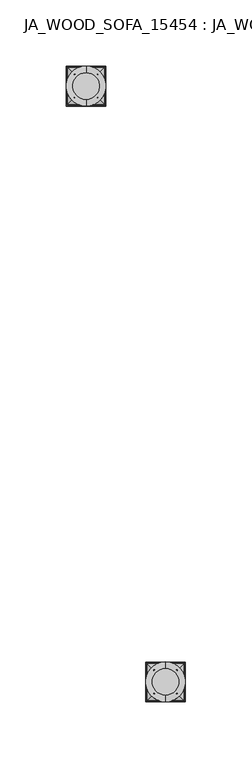
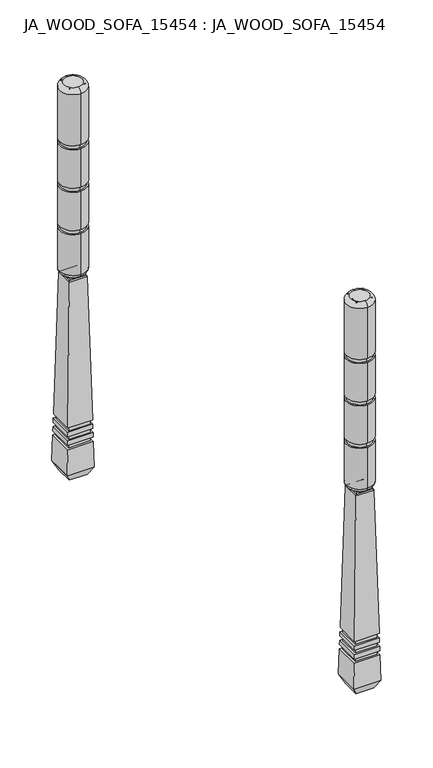
"""IFC4 building model written with IfcOpenShell, lengths in millimetres: furniture geometry, JA_WOOD_SOFA_15454 : JA_WOOD_SOFA_15454."""

from ifc_helpers import new_model, si_unit, point, frame, origin, origin_with_axes, place, context, project, spatial, polyline, circle_curve, ellipse_curve, trimmed, outline, extrude, faceted_brep, source, transform, mapped, element, save
from ifc_brep_helpers import plane_surface, cylinder_surface, revolved_surface, advanced_brep


def ja_wood_sofa_15454_ja_wood_sofa_15454_5725a5a5(model_context):
    return source(origin(), model_context, "Body", "SolidModel", [
        advanced_brep(
        [(237.5, 460.0, 460.0), (237.5, 440.0, 460.0), (237.5, 442.0710678, 235.0), (237.5, 457.9289322, 235.0), (237.5, 465.0, 245.0), (237.5, 465.0, 242.0710678), (237.5, 435.0, 242.0710678), (237.5, 435.0, 245.0), (237.5, 435.0, 290.0), (237.5, 465.0, 290.0), (237.5, 465.0, 455.0000045), (237.5, 465.0, 450.0), (237.5, 465.0, 395.0), (237.5, 435.0, 395.0), (237.5, 435.0, 450.0), (237.5, 435.0, 455.0000074), (237.5, 465.0, 390.0), (237.5, 465.0, 345.0), (237.5, 435.0, 345.0), (237.5, 435.0, 390.0), (237.5, 465.0, 340.0), (237.5, 465.0, 295.0), (237.5, 435.0, 295.0), (237.5, 435.0, 340.0), (237.5, 436.4644661, 238.5355339), (237.5, 463.5355339, 238.5355339), (237.5, 461.4644661, 236.4644661), (237.5, 438.5355339, 236.4644661), (237.5, 437.0, 340.0), (237.5, 437.0, 345.0), (237.5, 463.0, 345.0), (237.5, 463.0, 340.0), (237.5, 437.0, 390.0), (237.5, 437.0, 395.0), (237.5, 463.0, 395.0), (237.5, 463.0, 390.0), (237.5, 437.0, 290.0), (237.5, 437.0, 295.0), (237.5, 463.0, 295.0), (237.5, 463.0, 290.0)],
        [
            (0, 1, circle_curve(frame((237.5, 450.0, 460.0), z_axis=(0.0, 0.0, 1.0), x_axis=(0.0, 1.0, 0.0)), 10.0)),
            (1, 0, circle_curve(frame((237.5, 450.0, 460.0), z_axis=(0.0, 0.0, 1.0), x_axis=(0.0, -1.0, 0.0)), 10.0)),
            (2, 3, circle_curve(frame((237.5, 450.0, 235.0), z_axis=(0.0, 0.0, -1.0), x_axis=(0.0, 1.0, 0.0)), 7.9289322)),
            (3, 2, circle_curve(frame((237.5, 450.0, 235.0), z_axis=(0.0, 0.0, -1.0), x_axis=(0.0, -1.0, 0.0)), 7.9289322)),
            (4, 5),
            (5, 6, circle_curve(frame((237.5, 450.0, 242.0710678), z_axis=(0.0, 0.0, 1.0), x_axis=(0.0, -1.0, 0.0)), 15.0)),
            (6, 7),
            (7, 8),
            (8, 9, circle_curve(frame((237.5, 450.0, 290.0), z_axis=(0.0, 0.0, -1.0), x_axis=(0.0, -1.0, 0.0)), 15.0)),
            (9, 4),
            (10, 11),
            (11, 12),
            (12, 13, circle_curve(frame((237.5, 450.0, 395.0), z_axis=(0.0, 0.0, 1.0), x_axis=(0.0, -1.0, 0.0)), 15.0)),
            (13, 14),
            (14, 15),
            (15, 10, circle_curve(frame((237.5, 450.0, 455.0), z_axis=(0.0, 0.0, -1.0), x_axis=(0.0, -1.0, 0.0)), 15.0)),
            (16, 17),
            (17, 18, circle_curve(frame((237.5, 450.0, 345.0), z_axis=(0.0, 0.0, 1.0), x_axis=(0.0, -1.0, 0.0)), 15.0)),
            (18, 19),
            (19, 16, circle_curve(frame((237.5, 450.0, 390.0), z_axis=(0.0, 0.0, -1.0), x_axis=(0.0, -1.0, 0.0)), 15.0)),
            (20, 21),
            (21, 22, circle_curve(frame((237.5, 450.0, 295.0), z_axis=(0.0, 0.0, 1.0), x_axis=(0.0, -1.0, 0.0)), 15.0)),
            (22, 23),
            (23, 20, circle_curve(frame((237.5, 450.0, 340.0), z_axis=(0.0, 0.0, -1.0), x_axis=(0.0, -1.0, 0.0)), 15.0)),
            (9, 8, circle_curve(frame((237.5, 450.0, 290.0), z_axis=(0.0, 0.0, -1.0), x_axis=(0.0, -1.0, 0.0)), 15.0)),
            (6, 5, circle_curve(frame((237.5, 450.0, 242.0710678), z_axis=(0.0, 0.0, 1.0), x_axis=(0.0, -1.0, 0.0)), 15.0)),
            (10, 15, circle_curve(frame((237.5, 450.0, 455.0), z_axis=(0.0, 0.0, -1.0), x_axis=(0.0, -1.0, 0.0)), 15.0)),
            (13, 12, circle_curve(frame((237.5, 450.0, 395.0), z_axis=(0.0, 0.0, 1.0), x_axis=(0.0, -1.0, 0.0)), 15.0)),
            (16, 19, circle_curve(frame((237.5, 450.0, 390.0), z_axis=(0.0, 0.0, -1.0), x_axis=(0.0, -1.0, 0.0)), 15.0)),
            (18, 17, circle_curve(frame((237.5, 450.0, 345.0), z_axis=(0.0, 0.0, 1.0), x_axis=(0.0, -1.0, 0.0)), 15.0)),
            (20, 23, circle_curve(frame((237.5, 450.0, 340.0), z_axis=(0.0, 0.0, -1.0), x_axis=(0.0, -1.0, 0.0)), 15.0)),
            (22, 21, circle_curve(frame((237.5, 450.0, 295.0), z_axis=(0.0, 0.0, 1.0), x_axis=(0.0, -1.0, 0.0)), 15.0)),
            (24, 6, circle_curve(frame((237.5, 440.0, 242.0710678), z_axis=(-1.0, 0.0, 0.0), x_axis=(0.0, -1.0, 0.0)), 5.0)),
            (5, 25, circle_curve(frame((237.5, 460.0, 242.0710678), z_axis=(-1.0, 0.0, 0.0), x_axis=(0.0, 1.0, 0.0)), 5.0)),
            (25, 24, circle_curve(frame((237.5, 450.0, 238.5355339), z_axis=(0.0, 0.0, 1.0), x_axis=(0.0, 1.0, 0.0)), 13.5355339)),
            (25, 26),
            (26, 27, circle_curve(frame((237.5, 450.0, 236.4644661), z_axis=(0.0, 0.0, 1.0), x_axis=(0.0, 1.0, 0.0)), 11.4644661)),
            (27, 24),
            (26, 3, circle_curve(frame((237.5, 457.9289322, 240.0), z_axis=(-1.0, 0.0, 0.0), x_axis=(0.0, 1.0, 0.0)), 5.0)),
            (2, 27, circle_curve(frame((237.5, 442.0710678, 240.0), z_axis=(-1.0, 0.0, 0.0), x_axis=(0.0, -1.0, 0.0)), 5.0)),
            (24, 25, circle_curve(frame((237.5, 450.0, 238.5355339), z_axis=(0.0, 0.0, 1.0), x_axis=(0.0, -1.0, 0.0)), 13.5355339)),
            (27, 26, circle_curve(frame((237.5, 450.0, 236.4644661), z_axis=(0.0, 0.0, 1.0), x_axis=(0.0, -1.0, 0.0)), 11.4644661)),
            (15, 1, circle_curve(frame((237.5, 440.0, 455.0), z_axis=(-1.0, 0.0, 0.0), x_axis=(0.0, -1.0, 0.0)), 5.0)),
            (0, 10, circle_curve(frame((237.5, 460.0, 455.0), z_axis=(-1.0, 0.0, 0.0), x_axis=(0.0, 1.0, 0.0)), 5.0)),
            (28, 29),
            (29, 30, circle_curve(frame((237.5, 450.0, 345.0), z_axis=(0.0, 0.0, -1.0), x_axis=(0.0, 1.0, 0.0)), 13.0)),
            (30, 31),
            (31, 28, circle_curve(frame((237.5, 450.0, 340.0), z_axis=(0.0, 0.0, 1.0), x_axis=(0.0, 1.0, 0.0)), 13.0)),
            (32, 33),
            (33, 34, circle_curve(frame((237.5, 450.0, 395.0), z_axis=(0.0, 0.0, -1.0), x_axis=(0.0, 1.0, 0.0)), 13.0)),
            (34, 35),
            (35, 32, circle_curve(frame((237.5, 450.0, 390.0), z_axis=(0.0, 0.0, 1.0), x_axis=(0.0, 1.0, 0.0)), 13.0)),
            (36, 37),
            (37, 38, circle_curve(frame((237.5, 450.0, 295.0), z_axis=(0.0, 0.0, -1.0), x_axis=(0.0, 1.0, 0.0)), 13.0)),
            (38, 39),
            (39, 36, circle_curve(frame((237.5, 450.0, 290.0), z_axis=(0.0, 0.0, 1.0), x_axis=(0.0, 1.0, 0.0)), 13.0)),
            (28, 31, circle_curve(frame((237.5, 450.0, 340.0), z_axis=(0.0, 0.0, 1.0), x_axis=(0.0, -1.0, 0.0)), 13.0)),
            (30, 29, circle_curve(frame((237.5, 450.0, 345.0), z_axis=(0.0, 0.0, -1.0), x_axis=(0.0, -1.0, 0.0)), 13.0)),
            (32, 35, circle_curve(frame((237.5, 450.0, 390.0), z_axis=(0.0, 0.0, 1.0), x_axis=(0.0, -1.0, 0.0)), 13.0)),
            (34, 33, circle_curve(frame((237.5, 450.0, 395.0), z_axis=(0.0, 0.0, -1.0), x_axis=(0.0, -1.0, 0.0)), 13.0)),
            (36, 39, circle_curve(frame((237.5, 450.0, 290.0), z_axis=(0.0, 0.0, 1.0), x_axis=(0.0, -1.0, 0.0)), 13.0)),
            (38, 37, circle_curve(frame((237.5, 450.0, 295.0), z_axis=(0.0, 0.0, -1.0), x_axis=(0.0, -1.0, 0.0)), 13.0)),
        ],
        [
            plane_surface(frame((237.5, 435.0, 460.0), z_axis=(0.0, 0.0, 1.0), x_axis=(1.0, 0.0, 0.0))),
            plane_surface(frame((237.5, 435.0, 235.0), z_axis=(0.0, 0.0, -1.0), x_axis=(-1.0, 0.0, 0.0))),
            cylinder_surface(frame((237.5, 450.0, 235.0), z_axis=(0.0, 0.0, 1.0), x_axis=(0.0, -1.0, 0.0)), 15.0),
            revolved_surface(trimmed(ellipse_curve(frame((237.5, 460.0, 242.0710678), z_axis=(1.0, 0.0, 0.0), x_axis=(0.0, 1.0, 0.0)), 5.0, 5.0), [point((237.5, 463.5355339, 238.5355339))], [point((237.5, 465.0, 242.0710678))], True, "CARTESIAN"), (237.5, 450.0, 235.0), (0.0, 0.0, 1.0)),
            revolved_surface(polyline([(237.5, 461.4644661, 236.4644661), (237.5, 463.5355339, 238.5355339)]), (237.5, 450.0, 235.0), (0.0, 0.0, 1.0)),
            revolved_surface(trimmed(ellipse_curve(frame((237.5, 457.9289322, 240.0), z_axis=(1.0, 0.0, 0.0), x_axis=(0.0, 1.0, 0.0)), 5.0, 5.0), [point((237.5, 457.9289322, 235.0))], [point((237.5, 461.4644661, 236.4644661))], True, "CARTESIAN"), (237.5, 450.0, 235.0), (0.0, 0.0, 1.0)),
            revolved_surface(trimmed(ellipse_curve(frame((237.5, 440.0, 242.0710678), z_axis=(-1.0, 0.0, 0.0), x_axis=(0.0, -1.0, 0.0)), 5.0, 5.0), [point((237.5, 436.4644661, 238.5355339))], [point((237.5, 435.0, 242.0710678))], True, "CARTESIAN"), (237.5, 450.0, 235.0), (0.0, 0.0, 1.0)),
            revolved_surface(polyline([(237.5, 438.5355339, 236.4644661), (237.5, 436.4644661, 238.5355339)]), (237.5, 450.0, 235.0), (0.0, 0.0, 1.0)),
            revolved_surface(trimmed(ellipse_curve(frame((237.5, 442.0710678, 240.0), z_axis=(-1.0, 0.0, 0.0), x_axis=(0.0, -1.0, 0.0)), 5.0, 5.0), [point((237.5, 442.0710678, 235.0))], [point((237.5, 438.5355339, 236.4644661))], True, "CARTESIAN"), (237.5, 450.0, 235.0), (0.0, 0.0, 1.0)),
            revolved_surface(trimmed(ellipse_curve(frame((237.5, 460.0, 455.0), z_axis=(1.0, 0.0, 0.0), x_axis=(0.0, 1.0, 0.0)), 5.0, 5.0), [point((237.5, 465.0, 455.0))], [point((237.5, 460.0, 460.0))], True, "CARTESIAN"), (237.5, 450.0, 235.0), (0.0, 0.0, 1.0)),
            revolved_surface(trimmed(ellipse_curve(frame((237.5, 440.0, 455.0), z_axis=(-1.0, 0.0, 0.0), x_axis=(0.0, -1.0, 0.0)), 5.0, 5.0), [point((237.5, 435.0, 455.0))], [point((237.5, 440.0, 460.0))], True, "CARTESIAN"), (237.5, 450.0, 235.0), (0.0, 0.0, 1.0)),
            cylinder_surface(frame((237.5, 450.0, 235.0), z_axis=(0.0, 0.0, 1.0), x_axis=(0.0, 1.0, 0.0)), 13.0),
            cylinder_surface(frame((237.5, 450.0, 235.0), z_axis=(0.0, 0.0, 1.0), x_axis=(0.0, -1.0, 0.0)), 13.0),
            plane_surface(frame((237.5, 450.0, 340.0), z_axis=(0.0, 0.0, 1.0), x_axis=(0.0, -1.0, 0.0))),
            plane_surface(frame((237.5, 450.0, 345.0), z_axis=(0.0, 0.0, -1.0), x_axis=(0.0, -1.0, 0.0))),
            plane_surface(frame((237.5, 450.0, 390.0), z_axis=(0.0, 0.0, 1.0), x_axis=(0.0, -1.0, 0.0))),
            plane_surface(frame((237.5, 450.0, 395.0), z_axis=(0.0, 0.0, -1.0), x_axis=(0.0, -1.0, 0.0))),
            plane_surface(frame((237.5, 450.0, 290.0), z_axis=(0.0, 0.0, 1.0), x_axis=(0.0, -1.0, 0.0))),
            plane_surface(frame((237.5, 450.0, 295.0), z_axis=(0.0, 0.0, -1.0), x_axis=(0.0, -1.0, 0.0))),
        ],
        [
            (0, [[1, 2]]),
            (1, [[3, 4]]),
            (2, [[5, 6, 7, 8, 9, 10]]),
            (2, [[11, 12, 13, 14, 15, 16]]),
            (2, [[17, 18, 19, 20]]),
            (2, [[21, 22, 23, 24]]),
            (2, [[-5, -10, 25, -8, -7, 26]]),
            (2, [[-11, 27, -15, -14, 28, -12]]),
            (2, [[-17, 29, -19, 30]]),
            (2, [[-21, 31, -23, 32]]),
            (3, [[33, -6, 34, 35]]),
            (4, [[-35, 36, 37, 38]]),
            (5, [[-37, 39, -3, 40]]),
            (6, [[-33, 41, -34, -26]]),
            (7, [[-38, 42, -36, -41]]),
            (8, [[-40, -4, -39, -42]]),
            (9, [[43, -1, 44, -16]]),
            (10, [[-43, -27, -44, -2]]),
            (11, [[45, 46, 47, 48]]),
            (11, [[49, 50, 51, 52]]),
            (11, [[53, 54, 55, 56]]),
            (12, [[-45, 57, -47, 58]]),
            (13, [[-24, -31], [-48, -57]]),
            (14, [[-18, -30], [-46, -58]]),
            (12, [[-49, 59, -51, 60]]),
            (15, [[-20, -29], [-52, -59]]),
            (16, [[-13, -28], [-50, -60]]),
            (12, [[-53, 61, -55, 62]]),
            (17, [[-9, -25], [-56, -61]]),
            (18, [[-22, -32], [-54, -62]]),
        ],
    ),
        extrude(outline(polyline([(246.5, 459.0), (246.5, 441.0), (228.5, 441.0), (228.5, 459.0), (246.5, 459.0)])), origin_with_axes(), (0.0, 0.0, 1.0), 460.0),
        advanced_brep(
        [(223.7222222, 463.7777778, 65.0), (227.456543, 460.043457, 233.0444335), (247.543457, 460.043457, 233.0444335), (251.2777778, 463.7777778, 65.0), (247.543457, 439.956543, 233.0444335), (251.2777778, 436.2222222, 65.0), (227.456543, 439.956543, 233.0444335), (223.7222222, 436.2222222, 65.0), (252.5, 465.0, 10.0), (252.5, 435.0, 10.0), (222.5, 435.0, 10.0), (222.5, 465.0, 10.0), (232.5, 455.0, 10.0), (232.5, 445.0, 10.0), (242.5, 445.0, 10.0), (242.5, 455.0, 10.0), (225.5, 462.0, 60.0), (225.5, 462.0, 65.0), (249.5, 462.0, 65.0), (249.5, 462.0, 60.0), (223.5, 464.0, 55.0), (223.6111111, 463.8888889, 60.0), (251.3888889, 463.8888889, 60.0), (251.5, 464.0, 55.0), (225.5, 462.0, 50.0), (225.5, 462.0, 55.0), (249.5, 462.0, 55.0), (249.5, 462.0, 50.0), (223.2777778, 464.2222222, 45.0), (223.3888889, 464.1111111, 50.0), (251.6111111, 464.1111111, 50.0), (251.7222222, 464.2222222, 45.0), (225.5, 462.0, 40.0), (225.5, 462.0, 45.0), (249.5, 462.0, 45.0), (249.5, 462.0, 40.0), (223.1666667, 464.3333333, 40.0), (251.8333333, 464.3333333, 40.0), (249.5, 438.0, 65.0), (249.5, 438.0, 60.0), (251.3888889, 436.1111111, 60.0), (251.5, 436.0, 55.0), (249.5, 438.0, 55.0), (249.5, 438.0, 50.0), (251.6111111, 435.8888889, 50.0), (251.7222222, 435.7777778, 45.0), (249.5, 438.0, 45.0), (249.5, 438.0, 40.0), (251.8333333, 435.6666667, 40.0), (225.5, 438.0, 65.0), (225.5, 438.0, 60.0), (223.6111111, 436.1111111, 60.0), (223.5, 436.0, 55.0), (225.5, 438.0, 55.0), (225.5, 438.0, 50.0), (223.3888889, 435.8888889, 50.0), (223.2777778, 435.7777778, 45.0), (225.5, 438.0, 45.0), (225.5, 438.0, 40.0), (223.1666667, 435.6666667, 40.0), (232.5, 455.0, 235.0), (242.5, 455.0, 235.0), (229.4560493, 458.0439507, 235.0), (245.5439507, 458.0439507, 235.0), (242.5, 445.0, 235.0), (245.5439507, 441.9560493, 235.0), (232.5, 445.0, 235.0), (229.4560493, 441.9560493, 235.0)],
        [
            (0, 1),
            (1, 2),
            (2, 3),
            (3, 0),
            (2, 4),
            (4, 5),
            (5, 3),
            (4, 6),
            (6, 7),
            (7, 5),
            (6, 1),
            (0, 7),
            (8, 9),
            (9, 10),
            (10, 11),
            (11, 8),
            (12, 13),
            (13, 14),
            (14, 15),
            (15, 12),
            (16, 17),
            (17, 18),
            (18, 19),
            (19, 16),
            (20, 21),
            (21, 22),
            (22, 23),
            (23, 20),
            (24, 25),
            (25, 26),
            (26, 27),
            (27, 24),
            (28, 29),
            (29, 30),
            (30, 31),
            (31, 28),
            (32, 33),
            (33, 34),
            (34, 35),
            (35, 32),
            (11, 36),
            (36, 37),
            (37, 8),
            (18, 38),
            (38, 39),
            (39, 19),
            (22, 40),
            (40, 41),
            (41, 23),
            (26, 42),
            (42, 43),
            (43, 27),
            (30, 44),
            (44, 45),
            (45, 31),
            (34, 46),
            (46, 47),
            (47, 35),
            (37, 48),
            (48, 9),
            (38, 49),
            (49, 50),
            (50, 39),
            (40, 51),
            (51, 52),
            (52, 41),
            (42, 53),
            (53, 54),
            (54, 43),
            (44, 55),
            (55, 56),
            (56, 45),
            (46, 57),
            (57, 58),
            (58, 47),
            (48, 59),
            (59, 10),
            (17, 49),
            (16, 50),
            (21, 51),
            (20, 52),
            (25, 53),
            (24, 54),
            (29, 55),
            (28, 56),
            (33, 57),
            (32, 58),
            (36, 59),
            (60, 12),
            (15, 61),
            (61, 60),
            (1, 62, ellipse_curve(frame((229.4560493, 458.0439507, 233.0), z_axis=(0.7071067811865471, 0.7071067811865477, 0.0), x_axis=(-0.707106781186548, 0.707106781186547, 0.0)), 2.8284271, 2.0)),
            (62, 63),
            (63, 2, ellipse_curve(frame((245.5439507, 458.0439507, 233.0), z_axis=(-0.7071067811865476, 0.7071067811865474, 0.0), x_axis=(-0.7071067811865476, -0.7071067811865475, 0.0)), 2.8284271, 2.0)),
            (14, 64),
            (64, 61),
            (63, 65),
            (65, 4, ellipse_curve(frame((245.5439507, 441.9560493, 233.0), z_axis=(0.7071067811865475, 0.7071067811865476, 0.0), x_axis=(-0.7071067811865475, 0.7071067811865475, 0.0)), 2.8284271, 2.0)),
            (13, 66),
            (66, 64),
            (65, 67),
            (67, 6, ellipse_curve(frame((229.4560493, 441.9560493, 233.0), z_axis=(0.7071067811865477, -0.7071067811865472, 0.0), x_axis=(0.7071067811865474, 0.7071067811865476, 0.0)), 2.8284271, 2.0)),
            (60, 66),
            (62, 67),
        ],
        [
            plane_surface(frame((227.456543, 460.043457, 233.0444335), z_axis=(0.0, 0.99975317783161, 0.022216737285146875), x_axis=(1.0, 0.0, 0.0))),
            plane_surface(frame((247.543457, 460.043457, 233.0444335), z_axis=(0.99975317783161, 0.0, 0.022216737285146875), x_axis=(0.0, -1.0, 0.0))),
            plane_surface(frame((247.543457, 439.956543, 233.0444335), z_axis=(0.0, -0.99975317783161, 0.02221673728514687), x_axis=(-1.0, 0.0, 0.0))),
            plane_surface(frame((227.456543, 439.956543, 233.0444335), z_axis=(-0.99975317783161, 0.0, 0.022216737285146868), x_axis=(0.0, 1.0, 0.0))),
            plane_surface(frame((222.5, 435.0, 10.0), z_axis=(0.0, 0.0, -1.0), x_axis=(0.0, 1.0, 0.0))),
            plane_surface(frame((225.5, 462.0, 65.0), z_axis=(0.0, 1.0, 0.0), x_axis=(1.0, 0.0, 0.0))),
            plane_surface(frame((223.6111111, 463.8888889, 60.0), z_axis=(0.0, 0.99975317783161, 0.022216737285146875), x_axis=(1.0, 0.0, 0.0))),
            plane_surface(frame((225.5, 462.0, 55.0), z_axis=(0.0, 1.0, 0.0), x_axis=(1.0, 0.0, 0.0))),
            plane_surface(frame((223.3888889, 464.1111111, 50.0), z_axis=(0.0, 0.99975317783161, 0.022216737285146875), x_axis=(1.0, 0.0, 0.0))),
            plane_surface(frame((225.5, 462.0, 45.0), z_axis=(0.0, 1.0, 0.0), x_axis=(1.0, 0.0, 0.0))),
            plane_surface(frame((223.1666667, 464.3333333, 40.0), z_axis=(0.0, 0.99975317783161, 0.022216737285146875), x_axis=(1.0, 0.0, 0.0))),
            plane_surface(frame((249.5, 462.0, 65.0), z_axis=(1.0, 0.0, 0.0), x_axis=(0.0, -1.0, 0.0))),
            plane_surface(frame((251.3888889, 463.8888889, 60.0), z_axis=(0.99975317783161, 0.0, 0.022216737285146875), x_axis=(0.0, -1.0, 0.0))),
            plane_surface(frame((249.5, 462.0, 55.0), z_axis=(1.0, 0.0, 0.0), x_axis=(0.0, -1.0, 0.0))),
            plane_surface(frame((251.6111111, 464.1111111, 50.0), z_axis=(0.99975317783161, 0.0, 0.022216737285146875), x_axis=(0.0, -1.0, 0.0))),
            plane_surface(frame((249.5, 462.0, 45.0), z_axis=(1.0, 0.0, 0.0), x_axis=(0.0, -1.0, 0.0))),
            plane_surface(frame((251.8333333, 464.3333333, 40.0), z_axis=(0.99975317783161, 0.0, 0.022216737285146875), x_axis=(0.0, -1.0, 0.0))),
            plane_surface(frame((249.5, 438.0, 65.0), z_axis=(0.0, -1.0, 0.0), x_axis=(-1.0, 0.0, 0.0))),
            plane_surface(frame((251.3888889, 436.1111111, 60.0), z_axis=(0.0, -0.99975317783161, 0.02221673728514687), x_axis=(-1.0, 0.0, 0.0))),
            plane_surface(frame((249.5, 438.0, 55.0), z_axis=(0.0, -1.0, 0.0), x_axis=(-1.0, 0.0, 0.0))),
            plane_surface(frame((251.6111111, 435.8888889, 50.0), z_axis=(0.0, -0.99975317783161, 0.02221673728514687), x_axis=(-1.0, 0.0, 0.0))),
            plane_surface(frame((249.5, 438.0, 45.0), z_axis=(0.0, -1.0, 0.0), x_axis=(-1.0, 0.0, 0.0))),
            plane_surface(frame((251.8333333, 435.6666667, 40.0), z_axis=(0.0, -0.99975317783161, 0.02221673728514687), x_axis=(-1.0, 0.0, 0.0))),
            plane_surface(frame((223.7222222, 436.2222222, 65.0), z_axis=(0.0, 0.0, -1.0), x_axis=(0.0, 1.0, 0.0))),
            plane_surface(frame((225.5, 438.0, 65.0), z_axis=(-1.0, 0.0, 0.0), x_axis=(0.0, 1.0, 0.0))),
            plane_surface(frame((225.5, 438.0, 60.0), z_axis=(0.0, 0.0, 1.0), x_axis=(0.0, 1.0, 0.0))),
            plane_surface(frame((223.6111111, 436.1111111, 60.0), z_axis=(-0.99975317783161, 0.0, 0.022216737285146868), x_axis=(0.0, 1.0, 0.0))),
            plane_surface(frame((223.5, 436.0, 55.0), z_axis=(0.0, 0.0, -1.0), x_axis=(0.0, 1.0, 0.0))),
            plane_surface(frame((225.5, 438.0, 55.0), z_axis=(-1.0, 0.0, 0.0), x_axis=(0.0, 1.0, 0.0))),
            plane_surface(frame((225.5, 438.0, 50.0), z_axis=(0.0, 0.0, 1.0), x_axis=(0.0, 1.0, 0.0))),
            plane_surface(frame((223.3888889, 435.8888889, 50.0), z_axis=(-0.99975317783161, 0.0, 0.022216737285146868), x_axis=(0.0, 1.0, 0.0))),
            plane_surface(frame((223.2777778, 435.7777778, 45.0), z_axis=(0.0, 0.0, -1.0), x_axis=(0.0, 1.0, 0.0))),
            plane_surface(frame((225.5, 438.0, 45.0), z_axis=(-1.0, 0.0, 0.0), x_axis=(0.0, 1.0, 0.0))),
            plane_surface(frame((225.5, 438.0, 40.0), z_axis=(0.0, 0.0, 1.0), x_axis=(0.0, 1.0, 0.0))),
            plane_surface(frame((223.1666667, 435.6666667, 40.0), z_axis=(-0.99975317783161, 0.0, 0.022216737285146868), x_axis=(0.0, 1.0, 0.0))),
            plane_surface(frame((232.5, 455.0, 10.0), z_axis=(0.0, -1.0, 0.0), x_axis=(1.0, 0.0, 0.0))),
            cylinder_surface(frame((222.5, 458.0439507, 233.0), z_axis=(-1.0, 0.0, 0.0), x_axis=(0.0, 1.0, 0.0)), 2.0),
            plane_surface(frame((242.5, 455.0, 10.0), z_axis=(-1.0, 0.0, 0.0), x_axis=(0.0, -1.0, 0.0))),
            cylinder_surface(frame((245.5439507, 465.0, 233.0), z_axis=(0.0, 1.0, 0.0), x_axis=(1.0, 0.0, 0.0)), 2.0),
            plane_surface(frame((242.5, 445.0, 10.0), z_axis=(0.0, 1.0, 0.0), x_axis=(-1.0, 0.0, 0.0))),
            cylinder_surface(frame((252.5, 441.9560493, 233.0), z_axis=(1.0, 0.0, 0.0), x_axis=(0.0, -1.0, 0.0)), 2.0),
            plane_surface(frame((232.5, 445.0, 10.0), z_axis=(1.0, 0.0, 0.0), x_axis=(0.0, 1.0, 0.0))),
            plane_surface(frame((232.5, 445.0, 235.0), z_axis=(0.0, 0.0, 1.0), x_axis=(0.0, 1.0, 0.0))),
            cylinder_surface(frame((229.4560493, 435.0, 233.0), z_axis=(0.0, -1.0, 0.0), x_axis=(-1.0, 0.0, 0.0)), 2.0),
        ],
        [
            (0, [[1, 2, 3, 4]]),
            (1, [[-3, 5, 6, 7]]),
            (2, [[-6, 8, 9, 10]]),
            (3, [[-9, 11, -1, 12]]),
            (4, [[13, 14, 15, 16], [17, 18, 19, 20]]),
            (5, [[21, 22, 23, 24]]),
            (6, [[25, 26, 27, 28]]),
            (7, [[29, 30, 31, 32]]),
            (8, [[33, 34, 35, 36]]),
            (9, [[37, 38, 39, 40]]),
            (10, [[41, 42, 43, -16]]),
            (11, [[-23, 44, 45, 46]]),
            (12, [[-27, 47, 48, 49]]),
            (13, [[-31, 50, 51, 52]]),
            (14, [[-35, 53, 54, 55]]),
            (15, [[-39, 56, 57, 58]]),
            (16, [[-43, 59, 60, -13]]),
            (17, [[-45, 61, 62, 63]]),
            (18, [[-48, 64, 65, 66]]),
            (19, [[-51, 67, 68, 69]]),
            (20, [[-54, 70, 71, 72]]),
            (21, [[-57, 73, 74, 75]]),
            (22, [[-60, 76, 77, -14]]),
            (23, [[-7, -10, -12, -4], [78, -61, -44, -22]]),
            (24, [[-62, -78, -21, 79]]),
            (25, [[80, -64, -47, -26], [-46, -63, -79, -24]]),
            (26, [[-65, -80, -25, 81]]),
            (27, [[-49, -66, -81, -28], [82, -67, -50, -30]]),
            (28, [[-68, -82, -29, 83]]),
            (29, [[84, -70, -53, -34], [-52, -69, -83, -32]]),
            (30, [[-71, -84, -33, 85]]),
            (31, [[-55, -72, -85, -36], [86, -73, -56, -38]]),
            (32, [[-74, -86, -37, 87]]),
            (33, [[88, -76, -59, -42], [-58, -75, -87, -40]]),
            (34, [[-77, -88, -41, -15]]),
            (35, [[89, -20, 90, 91]]),
            (36, [[92, 93, 94, -2]]),
            (37, [[-90, -19, 95, 96]]),
            (38, [[-94, 97, 98, -5]]),
            (39, [[-95, -18, 99, 100]]),
            (40, [[-98, 101, 102, -8]]),
            (41, [[-99, -17, -89, 103]]),
            (42, [[104, -101, -97, -93], [-96, -100, -103, -91]]),
            (43, [[-102, -104, -92, -11]]),
        ],
    ),
        faceted_brep([(252.5, 435.0, 10.0), (252.5, 465.0, 10.0), (222.5, 465.0, 10.0), (222.5, 435.0, 10.0), (247.5, 440.0, 0.0), (227.5, 440.0, 0.0), (227.5, 460.0, 0.0), (247.5, 460.0, 0.0)], [[[0, 1, 2, 3]], [[4, 5, 6, 7]], [[4, 7, 1, 0]], [[7, 6, 2, 1]], [[6, 5, 3, 2]], [[5, 4, 0, 3]]]),
        advanced_brep(
        [(297.5, 10.0, 460.0), (297.5, -10.0, 460.0), (297.5, -7.9289322, 235.0), (297.5, 7.9289322, 235.0), (297.5, 15.0, 245.0), (297.5, 15.0, 242.0710678), (297.5, -15.0, 242.0710678), (297.5, -15.0, 245.0), (297.5, -15.0, 290.0), (297.5, 15.0, 290.0), (297.5, 15.0, 455.0000045), (297.5, 15.0, 450.0), (297.5, 15.0, 395.0), (297.5, -15.0, 395.0), (297.5, -15.0, 450.0), (297.5, -15.0, 455.0000074), (297.5, 15.0, 390.0), (297.5, 15.0, 345.0), (297.5, -15.0, 345.0), (297.5, -15.0, 390.0), (297.5, 15.0, 340.0), (297.5, 15.0, 295.0), (297.5, -15.0, 295.0), (297.5, -15.0, 340.0), (297.5, -13.5355339, 238.5355339), (297.5, 13.5355339, 238.5355339), (297.5, 11.4644661, 236.4644661), (297.5, -11.4644661, 236.4644661), (297.5, -13.0, 340.0), (297.5, -13.0, 345.0), (297.5, 13.0, 345.0), (297.5, 13.0, 340.0), (297.5, -13.0, 390.0), (297.5, -13.0, 395.0), (297.5, 13.0, 395.0), (297.5, 13.0, 390.0), (297.5, -13.0, 290.0), (297.5, -13.0, 295.0), (297.5, 13.0, 295.0), (297.5, 13.0, 290.0)],
        [
            (0, 1, circle_curve(frame((297.5, 0.0, 460.0), z_axis=(0.0, 0.0, 1.0), x_axis=(0.0, 1.0, 0.0)), 10.0)),
            (1, 0, circle_curve(frame((297.5, 0.0, 460.0), z_axis=(0.0, 0.0, 1.0), x_axis=(0.0, -1.0, 0.0)), 10.0)),
            (2, 3, circle_curve(frame((297.5, 0.0, 235.0), z_axis=(0.0, 0.0, -1.0), x_axis=(0.0, 1.0, 0.0)), 7.9289322)),
            (3, 2, circle_curve(frame((297.5, 0.0, 235.0), z_axis=(0.0, 0.0, -1.0), x_axis=(0.0, -1.0, 0.0)), 7.9289322)),
            (4, 5),
            (5, 6, circle_curve(frame((297.5, 0.0, 242.0710678), z_axis=(0.0, 0.0, 1.0), x_axis=(0.0, -1.0, 0.0)), 15.0)),
            (6, 7),
            (7, 8),
            (8, 9, circle_curve(frame((297.5, 0.0, 290.0), z_axis=(0.0, 0.0, -1.0), x_axis=(0.0, -1.0, 0.0)), 15.0)),
            (9, 4),
            (10, 11),
            (11, 12),
            (12, 13, circle_curve(frame((297.5, 0.0, 395.0), z_axis=(0.0, 0.0, 1.0), x_axis=(0.0, -1.0, 0.0)), 15.0)),
            (13, 14),
            (14, 15),
            (15, 10, circle_curve(frame((297.5, 0.0, 455.0), z_axis=(0.0, 0.0, -1.0), x_axis=(0.0, -1.0, 0.0)), 15.0)),
            (16, 17),
            (17, 18, circle_curve(frame((297.5, 0.0, 345.0), z_axis=(0.0, 0.0, 1.0), x_axis=(0.0, -1.0, 0.0)), 15.0)),
            (18, 19),
            (19, 16, circle_curve(frame((297.5, 0.0, 390.0), z_axis=(0.0, 0.0, -1.0), x_axis=(0.0, -1.0, 0.0)), 15.0)),
            (20, 21),
            (21, 22, circle_curve(frame((297.5, 0.0, 295.0), z_axis=(0.0, 0.0, 1.0), x_axis=(0.0, -1.0, 0.0)), 15.0)),
            (22, 23),
            (23, 20, circle_curve(frame((297.5, 0.0, 340.0), z_axis=(0.0, 0.0, -1.0), x_axis=(0.0, -1.0, 0.0)), 15.0)),
            (9, 8, circle_curve(frame((297.5, 0.0, 290.0), z_axis=(0.0, 0.0, -1.0), x_axis=(0.0, -1.0, 0.0)), 15.0)),
            (6, 5, circle_curve(frame((297.5, 0.0, 242.0710678), z_axis=(0.0, 0.0, 1.0), x_axis=(0.0, -1.0, 0.0)), 15.0)),
            (10, 15, circle_curve(frame((297.5, 0.0, 455.0), z_axis=(0.0, 0.0, -1.0), x_axis=(0.0, -1.0, 0.0)), 15.0)),
            (13, 12, circle_curve(frame((297.5, 0.0, 395.0), z_axis=(0.0, 0.0, 1.0), x_axis=(0.0, -1.0, 0.0)), 15.0)),
            (16, 19, circle_curve(frame((297.5, 0.0, 390.0), z_axis=(0.0, 0.0, -1.0), x_axis=(0.0, -1.0, 0.0)), 15.0)),
            (18, 17, circle_curve(frame((297.5, 0.0, 345.0), z_axis=(0.0, 0.0, 1.0), x_axis=(0.0, -1.0, 0.0)), 15.0)),
            (20, 23, circle_curve(frame((297.5, 0.0, 340.0), z_axis=(0.0, 0.0, -1.0), x_axis=(0.0, -1.0, 0.0)), 15.0)),
            (22, 21, circle_curve(frame((297.5, 0.0, 295.0), z_axis=(0.0, 0.0, 1.0), x_axis=(0.0, -1.0, 0.0)), 15.0)),
            (24, 6, circle_curve(frame((297.5, -10.0, 242.0710678), z_axis=(-1.0, 0.0, 0.0), x_axis=(0.0, -1.0, 0.0)), 5.0)),
            (5, 25, circle_curve(frame((297.5, 10.0, 242.0710678), z_axis=(-1.0, 0.0, 0.0), x_axis=(0.0, 1.0, 0.0)), 5.0)),
            (25, 24, circle_curve(frame((297.5, 0.0, 238.5355339), z_axis=(0.0, 0.0, 1.0), x_axis=(0.0, 1.0, 0.0)), 13.5355339)),
            (25, 26),
            (26, 27, circle_curve(frame((297.5, 0.0, 236.4644661), z_axis=(0.0, 0.0, 1.0), x_axis=(0.0, 1.0, 0.0)), 11.4644661)),
            (27, 24),
            (26, 3, circle_curve(frame((297.5, 7.9289322, 240.0), z_axis=(-1.0, 0.0, 0.0), x_axis=(0.0, 1.0, 0.0)), 5.0)),
            (2, 27, circle_curve(frame((297.5, -7.9289322, 240.0), z_axis=(-1.0, 0.0, 0.0), x_axis=(0.0, -1.0, 0.0)), 5.0)),
            (24, 25, circle_curve(frame((297.5, 0.0, 238.5355339), z_axis=(0.0, 0.0, 1.0), x_axis=(0.0, -1.0, 0.0)), 13.5355339)),
            (27, 26, circle_curve(frame((297.5, 0.0, 236.4644661), z_axis=(0.0, 0.0, 1.0), x_axis=(0.0, -1.0, 0.0)), 11.4644661)),
            (15, 1, circle_curve(frame((297.5, -10.0, 455.0), z_axis=(-1.0, 0.0, 0.0), x_axis=(0.0, -1.0, 0.0)), 5.0)),
            (0, 10, circle_curve(frame((297.5, 10.0, 455.0), z_axis=(-1.0, 0.0, 0.0), x_axis=(0.0, 1.0, 0.0)), 5.0)),
            (28, 29),
            (29, 30, circle_curve(frame((297.5, 0.0, 345.0), z_axis=(0.0, 0.0, -1.0), x_axis=(0.0, 1.0, 0.0)), 13.0)),
            (30, 31),
            (31, 28, circle_curve(frame((297.5, 0.0, 340.0), z_axis=(0.0, 0.0, 1.0), x_axis=(0.0, 1.0, 0.0)), 13.0)),
            (32, 33),
            (33, 34, circle_curve(frame((297.5, 0.0, 395.0), z_axis=(0.0, 0.0, -1.0), x_axis=(0.0, 1.0, 0.0)), 13.0)),
            (34, 35),
            (35, 32, circle_curve(frame((297.5, 0.0, 390.0), z_axis=(0.0, 0.0, 1.0), x_axis=(0.0, 1.0, 0.0)), 13.0)),
            (36, 37),
            (37, 38, circle_curve(frame((297.5, 0.0, 295.0), z_axis=(0.0, 0.0, -1.0), x_axis=(0.0, 1.0, 0.0)), 13.0)),
            (38, 39),
            (39, 36, circle_curve(frame((297.5, 0.0, 290.0), z_axis=(0.0, 0.0, 1.0), x_axis=(0.0, 1.0, 0.0)), 13.0)),
            (28, 31, circle_curve(frame((297.5, 0.0, 340.0), z_axis=(0.0, 0.0, 1.0), x_axis=(0.0, -1.0, 0.0)), 13.0)),
            (30, 29, circle_curve(frame((297.5, 0.0, 345.0), z_axis=(0.0, 0.0, -1.0), x_axis=(0.0, -1.0, 0.0)), 13.0)),
            (32, 35, circle_curve(frame((297.5, 0.0, 390.0), z_axis=(0.0, 0.0, 1.0), x_axis=(0.0, -1.0, 0.0)), 13.0)),
            (34, 33, circle_curve(frame((297.5, 0.0, 395.0), z_axis=(0.0, 0.0, -1.0), x_axis=(0.0, -1.0, 0.0)), 13.0)),
            (36, 39, circle_curve(frame((297.5, 0.0, 290.0), z_axis=(0.0, 0.0, 1.0), x_axis=(0.0, -1.0, 0.0)), 13.0)),
            (38, 37, circle_curve(frame((297.5, 0.0, 295.0), z_axis=(0.0, 0.0, -1.0), x_axis=(0.0, -1.0, 0.0)), 13.0)),
        ],
        [
            plane_surface(frame((297.5, -15.0, 460.0), z_axis=(0.0, 0.0, 1.0), x_axis=(1.0, 0.0, 0.0))),
            plane_surface(frame((297.5, -15.0, 235.0), z_axis=(0.0, 0.0, -1.0), x_axis=(-1.0, 0.0, 0.0))),
            cylinder_surface(frame((297.5, 0.0, 235.0), z_axis=(0.0, 0.0, 1.0), x_axis=(0.0, -1.0, 0.0)), 15.0),
            revolved_surface(trimmed(ellipse_curve(frame((297.5, 10.0, 242.0710678), z_axis=(1.0, 0.0, 0.0), x_axis=(0.0, 1.0, 0.0)), 5.0, 5.0), [point((297.5, 13.5355339, 238.5355339))], [point((297.5, 15.0, 242.0710678))], True, "CARTESIAN"), (297.5, 0.0, 235.0), (0.0, 0.0, 1.0)),
            revolved_surface(polyline([(297.5, 11.4644661, 236.4644661), (297.5, 13.5355339, 238.5355339)]), (297.5, 0.0, 235.0), (0.0, 0.0, 1.0)),
            revolved_surface(trimmed(ellipse_curve(frame((297.5, 7.9289322, 240.0), z_axis=(1.0, 0.0, 0.0), x_axis=(0.0, 1.0, 0.0)), 5.0, 5.0), [point((297.5, 7.9289322, 235.0))], [point((297.5, 11.4644661, 236.4644661))], True, "CARTESIAN"), (297.5, 0.0, 235.0), (0.0, 0.0, 1.0)),
            revolved_surface(trimmed(ellipse_curve(frame((297.5, -10.0, 242.0710678), z_axis=(-1.0, 0.0, 0.0), x_axis=(0.0, -1.0, 0.0)), 5.0, 5.0), [point((297.5, -13.5355339, 238.5355339))], [point((297.5, -15.0, 242.0710678))], True, "CARTESIAN"), (297.5, 0.0, 235.0), (0.0, 0.0, 1.0)),
            revolved_surface(polyline([(297.5, -11.4644661, 236.4644661), (297.5, -13.5355339, 238.5355339)]), (297.5, 0.0, 235.0), (0.0, 0.0, 1.0)),
            revolved_surface(trimmed(ellipse_curve(frame((297.5, -7.9289322, 240.0), z_axis=(-1.0, 0.0, 0.0), x_axis=(0.0, -1.0, 0.0)), 5.0, 5.0), [point((297.5, -7.9289322, 235.0))], [point((297.5, -11.4644661, 236.4644661))], True, "CARTESIAN"), (297.5, 0.0, 235.0), (0.0, 0.0, 1.0)),
            revolved_surface(trimmed(ellipse_curve(frame((297.5, 10.0, 455.0), z_axis=(1.0, 0.0, 0.0), x_axis=(0.0, 1.0, 0.0)), 5.0, 5.0), [point((297.5, 15.0, 455.0))], [point((297.5, 10.0, 460.0))], True, "CARTESIAN"), (297.5, 0.0, 235.0), (0.0, 0.0, 1.0)),
            revolved_surface(trimmed(ellipse_curve(frame((297.5, -10.0, 455.0), z_axis=(-1.0, 0.0, 0.0), x_axis=(0.0, -1.0, 0.0)), 5.0, 5.0), [point((297.5, -15.0, 455.0))], [point((297.5, -10.0, 460.0))], True, "CARTESIAN"), (297.5, 0.0, 235.0), (0.0, 0.0, 1.0)),
            cylinder_surface(frame((297.5, 0.0, 235.0), z_axis=(0.0, 0.0, 1.0), x_axis=(0.0, 1.0, 0.0)), 13.0),
            cylinder_surface(frame((297.5, 0.0, 235.0), z_axis=(0.0, 0.0, 1.0), x_axis=(0.0, -1.0, 0.0)), 13.0),
            plane_surface(frame((297.5, 0.0, 340.0), z_axis=(0.0, 0.0, 1.0), x_axis=(0.0, -1.0, 0.0))),
            plane_surface(frame((297.5, 0.0, 345.0), z_axis=(0.0, 0.0, -1.0), x_axis=(0.0, -1.0, 0.0))),
            plane_surface(frame((297.5, 0.0, 390.0), z_axis=(0.0, 0.0, 1.0), x_axis=(0.0, -1.0, 0.0))),
            plane_surface(frame((297.5, 0.0, 395.0), z_axis=(0.0, 0.0, -1.0), x_axis=(0.0, -1.0, 0.0))),
            plane_surface(frame((297.5, 0.0, 290.0), z_axis=(0.0, 0.0, 1.0), x_axis=(0.0, -1.0, 0.0))),
            plane_surface(frame((297.5, 0.0, 295.0), z_axis=(0.0, 0.0, -1.0), x_axis=(0.0, -1.0, 0.0))),
        ],
        [
            (0, [[1, 2]]),
            (1, [[3, 4]]),
            (2, [[5, 6, 7, 8, 9, 10]]),
            (2, [[11, 12, 13, 14, 15, 16]]),
            (2, [[17, 18, 19, 20]]),
            (2, [[21, 22, 23, 24]]),
            (2, [[-5, -10, 25, -8, -7, 26]]),
            (2, [[-11, 27, -15, -14, 28, -12]]),
            (2, [[-17, 29, -19, 30]]),
            (2, [[-21, 31, -23, 32]]),
            (3, [[33, -6, 34, 35]]),
            (4, [[-35, 36, 37, 38]]),
            (5, [[-37, 39, -3, 40]]),
            (6, [[-33, 41, -34, -26]]),
            (7, [[-38, 42, -36, -41]]),
            (8, [[-40, -4, -39, -42]]),
            (9, [[43, -1, 44, -16]]),
            (10, [[-43, -27, -44, -2]]),
            (11, [[45, 46, 47, 48]]),
            (11, [[49, 50, 51, 52]]),
            (11, [[53, 54, 55, 56]]),
            (12, [[-45, 57, -47, 58]]),
            (13, [[-24, -31], [-48, -57]]),
            (14, [[-18, -30], [-46, -58]]),
            (12, [[-49, 59, -51, 60]]),
            (15, [[-20, -29], [-52, -59]]),
            (16, [[-13, -28], [-50, -60]]),
            (12, [[-53, 61, -55, 62]]),
            (17, [[-9, -25], [-56, -61]]),
            (18, [[-22, -32], [-54, -62]]),
        ],
    ),
        extrude(outline(polyline([(306.5, 9.0), (306.5, -9.0), (288.5, -9.0), (288.5, 9.0), (306.5, 9.0)])), origin_with_axes(), (0.0, 0.0, 1.0), 460.0),
        advanced_brep(
        [(283.7222222, 13.7777778, 65.0), (287.456543, 10.043457, 233.0444335), (307.543457, 10.043457, 233.0444335), (311.2777778, 13.7777778, 65.0), (307.543457, -10.043457, 233.0444335), (311.2777778, -13.7777778, 65.0), (287.456543, -10.043457, 233.0444335), (283.7222222, -13.7777778, 65.0), (312.5, 15.0, 10.0), (312.5, -15.0, 10.0), (282.5, -15.0, 10.0), (282.5, 15.0, 10.0), (292.5, 5.0, 10.0), (292.5, -5.0, 10.0), (302.5, -5.0, 10.0), (302.5, 5.0, 10.0), (285.5, 12.0, 60.0), (285.5, 12.0, 65.0), (309.5, 12.0, 65.0), (309.5, 12.0, 60.0), (283.5, 14.0, 55.0), (283.6111111, 13.8888889, 60.0), (311.3888889, 13.8888889, 60.0), (311.5, 14.0, 55.0), (285.5, 12.0, 50.0), (285.5, 12.0, 55.0), (309.5, 12.0, 55.0), (309.5, 12.0, 50.0), (283.2777778, 14.2222222, 45.0), (283.3888889, 14.1111111, 50.0), (311.6111111, 14.1111111, 50.0), (311.7222222, 14.2222222, 45.0), (285.5, 12.0, 40.0), (285.5, 12.0, 45.0), (309.5, 12.0, 45.0), (309.5, 12.0, 40.0), (283.1666667, 14.3333333, 40.0), (311.8333333, 14.3333333, 40.0), (309.5, -12.0, 65.0), (309.5, -12.0, 60.0), (311.3888889, -13.8888889, 60.0), (311.5, -14.0, 55.0), (309.5, -12.0, 55.0), (309.5, -12.0, 50.0), (311.6111111, -14.1111111, 50.0), (311.7222222, -14.2222222, 45.0), (309.5, -12.0, 45.0), (309.5, -12.0, 40.0), (311.8333333, -14.3333333, 40.0), (285.5, -12.0, 65.0), (285.5, -12.0, 60.0), (283.6111111, -13.8888889, 60.0), (283.5, -14.0, 55.0), (285.5, -12.0, 55.0), (285.5, -12.0, 50.0), (283.3888889, -14.1111111, 50.0), (283.2777778, -14.2222222, 45.0), (285.5, -12.0, 45.0), (285.5, -12.0, 40.0), (283.1666667, -14.3333333, 40.0), (292.5, 5.0, 235.0), (302.5, 5.0, 235.0), (289.4560493, 8.0439507, 235.0), (305.5439507, 8.0439507, 235.0), (302.5, -5.0, 235.0), (305.5439507, -8.0439507, 235.0), (292.5, -5.0, 235.0), (289.4560493, -8.0439507, 235.0)],
        [
            (0, 1),
            (1, 2),
            (2, 3),
            (3, 0),
            (2, 4),
            (4, 5),
            (5, 3),
            (4, 6),
            (6, 7),
            (7, 5),
            (6, 1),
            (0, 7),
            (8, 9),
            (9, 10),
            (10, 11),
            (11, 8),
            (12, 13),
            (13, 14),
            (14, 15),
            (15, 12),
            (16, 17),
            (17, 18),
            (18, 19),
            (19, 16),
            (20, 21),
            (21, 22),
            (22, 23),
            (23, 20),
            (24, 25),
            (25, 26),
            (26, 27),
            (27, 24),
            (28, 29),
            (29, 30),
            (30, 31),
            (31, 28),
            (32, 33),
            (33, 34),
            (34, 35),
            (35, 32),
            (11, 36),
            (36, 37),
            (37, 8),
            (18, 38),
            (38, 39),
            (39, 19),
            (22, 40),
            (40, 41),
            (41, 23),
            (26, 42),
            (42, 43),
            (43, 27),
            (30, 44),
            (44, 45),
            (45, 31),
            (34, 46),
            (46, 47),
            (47, 35),
            (37, 48),
            (48, 9),
            (38, 49),
            (49, 50),
            (50, 39),
            (40, 51),
            (51, 52),
            (52, 41),
            (42, 53),
            (53, 54),
            (54, 43),
            (44, 55),
            (55, 56),
            (56, 45),
            (46, 57),
            (57, 58),
            (58, 47),
            (48, 59),
            (59, 10),
            (17, 49),
            (16, 50),
            (21, 51),
            (20, 52),
            (25, 53),
            (24, 54),
            (29, 55),
            (28, 56),
            (33, 57),
            (32, 58),
            (36, 59),
            (60, 12),
            (15, 61),
            (61, 60),
            (1, 62, ellipse_curve(frame((289.4560493, 8.0439507, 233.0), z_axis=(0.7071067811865471, 0.7071067811865477, 0.0), x_axis=(-0.707106781186548, 0.707106781186547, 0.0)), 2.8284271, 2.0)),
            (62, 63),
            (63, 2, ellipse_curve(frame((305.5439507, 8.0439507, 233.0), z_axis=(-0.7071067811865476, 0.7071067811865474, 0.0), x_axis=(-0.7071067811865476, -0.7071067811865475, 0.0)), 2.8284271, 2.0)),
            (14, 64),
            (64, 61),
            (63, 65),
            (65, 4, ellipse_curve(frame((305.5439507, -8.0439507, 233.0), z_axis=(0.7071067811865475, 0.7071067811865476, 0.0), x_axis=(-0.7071067811865475, 0.7071067811865475, 0.0)), 2.8284271, 2.0)),
            (13, 66),
            (66, 64),
            (65, 67),
            (67, 6, ellipse_curve(frame((289.4560493, -8.0439507, 233.0), z_axis=(0.7071067811865477, -0.7071067811865472, 0.0), x_axis=(0.7071067811865474, 0.7071067811865476, 0.0)), 2.8284271, 2.0)),
            (60, 66),
            (62, 67),
        ],
        [
            plane_surface(frame((287.456543, 10.043457, 233.0444335), z_axis=(0.0, 0.99975317783161, 0.022216737285146875), x_axis=(1.0, 0.0, 0.0))),
            plane_surface(frame((307.543457, 10.043457, 233.0444335), z_axis=(0.99975317783161, 0.0, 0.022216737285146875), x_axis=(0.0, -1.0, 0.0))),
            plane_surface(frame((307.543457, -10.043457, 233.0444335), z_axis=(0.0, -0.99975317783161, 0.02221673728514687), x_axis=(-1.0, 0.0, 0.0))),
            plane_surface(frame((287.456543, -10.043457, 233.0444335), z_axis=(-0.99975317783161, 0.0, 0.022216737285146868), x_axis=(0.0, 1.0, 0.0))),
            plane_surface(frame((282.5, -15.0, 10.0), z_axis=(0.0, 0.0, -1.0), x_axis=(0.0, 1.0, 0.0))),
            plane_surface(frame((285.5, 12.0, 65.0), z_axis=(0.0, 1.0, 0.0), x_axis=(1.0, 0.0, 0.0))),
            plane_surface(frame((283.6111111, 13.8888889, 60.0), z_axis=(0.0, 0.99975317783161, 0.022216737285146875), x_axis=(1.0, 0.0, 0.0))),
            plane_surface(frame((285.5, 12.0, 55.0), z_axis=(0.0, 1.0, 0.0), x_axis=(1.0, 0.0, 0.0))),
            plane_surface(frame((283.3888889, 14.1111111, 50.0), z_axis=(0.0, 0.99975317783161, 0.022216737285146875), x_axis=(1.0, 0.0, 0.0))),
            plane_surface(frame((285.5, 12.0, 45.0), z_axis=(0.0, 1.0, 0.0), x_axis=(1.0, 0.0, 0.0))),
            plane_surface(frame((283.1666667, 14.3333333, 40.0), z_axis=(0.0, 0.99975317783161, 0.022216737285146875), x_axis=(1.0, 0.0, 0.0))),
            plane_surface(frame((309.5, 12.0, 65.0), z_axis=(1.0, 0.0, 0.0), x_axis=(0.0, -1.0, 0.0))),
            plane_surface(frame((311.3888889, 13.8888889, 60.0), z_axis=(0.99975317783161, 0.0, 0.022216737285146875), x_axis=(0.0, -1.0, 0.0))),
            plane_surface(frame((309.5, 12.0, 55.0), z_axis=(1.0, 0.0, 0.0), x_axis=(0.0, -1.0, 0.0))),
            plane_surface(frame((311.6111111, 14.1111111, 50.0), z_axis=(0.99975317783161, 0.0, 0.022216737285146875), x_axis=(0.0, -1.0, 0.0))),
            plane_surface(frame((309.5, 12.0, 45.0), z_axis=(1.0, 0.0, 0.0), x_axis=(0.0, -1.0, 0.0))),
            plane_surface(frame((311.8333333, 14.3333333, 40.0), z_axis=(0.99975317783161, 0.0, 0.022216737285146875), x_axis=(0.0, -1.0, 0.0))),
            plane_surface(frame((309.5, -12.0, 65.0), z_axis=(0.0, -1.0, 0.0), x_axis=(-1.0, 0.0, 0.0))),
            plane_surface(frame((311.3888889, -13.8888889, 60.0), z_axis=(0.0, -0.99975317783161, 0.02221673728514687), x_axis=(-1.0, 0.0, 0.0))),
            plane_surface(frame((309.5, -12.0, 55.0), z_axis=(0.0, -1.0, 0.0), x_axis=(-1.0, 0.0, 0.0))),
            plane_surface(frame((311.6111111, -14.1111111, 50.0), z_axis=(0.0, -0.99975317783161, 0.02221673728514687), x_axis=(-1.0, 0.0, 0.0))),
            plane_surface(frame((309.5, -12.0, 45.0), z_axis=(0.0, -1.0, 0.0), x_axis=(-1.0, 0.0, 0.0))),
            plane_surface(frame((311.8333333, -14.3333333, 40.0), z_axis=(0.0, -0.99975317783161, 0.02221673728514687), x_axis=(-1.0, 0.0, 0.0))),
            plane_surface(frame((283.7222222, -13.7777778, 65.0), z_axis=(0.0, 0.0, -1.0), x_axis=(0.0, 1.0, 0.0))),
            plane_surface(frame((285.5, -12.0, 65.0), z_axis=(-1.0, 0.0, 0.0), x_axis=(0.0, 1.0, 0.0))),
            plane_surface(frame((285.5, -12.0, 60.0), z_axis=(0.0, 0.0, 1.0), x_axis=(0.0, 1.0, 0.0))),
            plane_surface(frame((283.6111111, -13.8888889, 60.0), z_axis=(-0.99975317783161, 0.0, 0.022216737285146868), x_axis=(0.0, 1.0, 0.0))),
            plane_surface(frame((283.5, -14.0, 55.0), z_axis=(0.0, 0.0, -1.0), x_axis=(0.0, 1.0, 0.0))),
            plane_surface(frame((285.5, -12.0, 55.0), z_axis=(-1.0, 0.0, 0.0), x_axis=(0.0, 1.0, 0.0))),
            plane_surface(frame((285.5, -12.0, 50.0), z_axis=(0.0, 0.0, 1.0), x_axis=(0.0, 1.0, 0.0))),
            plane_surface(frame((283.3888889, -14.1111111, 50.0), z_axis=(-0.99975317783161, 0.0, 0.022216737285146868), x_axis=(0.0, 1.0, 0.0))),
            plane_surface(frame((283.2777778, -14.2222222, 45.0), z_axis=(0.0, 0.0, -1.0), x_axis=(0.0, 1.0, 0.0))),
            plane_surface(frame((285.5, -12.0, 45.0), z_axis=(-1.0, 0.0, 0.0), x_axis=(0.0, 1.0, 0.0))),
            plane_surface(frame((285.5, -12.0, 40.0), z_axis=(0.0, 0.0, 1.0), x_axis=(0.0, 1.0, 0.0))),
            plane_surface(frame((283.1666667, -14.3333333, 40.0), z_axis=(-0.99975317783161, 0.0, 0.022216737285146868), x_axis=(0.0, 1.0, 0.0))),
            plane_surface(frame((292.5, 5.0, 10.0), z_axis=(0.0, -1.0, 0.0), x_axis=(1.0, 0.0, 0.0))),
            cylinder_surface(frame((282.5, 8.0439507, 233.0), z_axis=(-1.0, 0.0, 0.0), x_axis=(0.0, 1.0, 0.0)), 2.0),
            plane_surface(frame((302.5, 5.0, 10.0), z_axis=(-1.0, 0.0, 0.0), x_axis=(0.0, -1.0, 0.0))),
            cylinder_surface(frame((305.5439507, 15.0, 233.0), z_axis=(0.0, 1.0, 0.0), x_axis=(1.0, 0.0, 0.0)), 2.0),
            plane_surface(frame((302.5, -5.0, 10.0), z_axis=(0.0, 1.0, 0.0), x_axis=(-1.0, 0.0, 0.0))),
            cylinder_surface(frame((312.5, -8.0439507, 233.0), z_axis=(1.0, 0.0, 0.0), x_axis=(0.0, -1.0, 0.0)), 2.0),
            plane_surface(frame((292.5, -5.0, 10.0), z_axis=(1.0, 0.0, 0.0), x_axis=(0.0, 1.0, 0.0))),
            plane_surface(frame((292.5, -5.0, 235.0), z_axis=(0.0, 0.0, 1.0), x_axis=(0.0, 1.0, 0.0))),
            cylinder_surface(frame((289.4560493, -15.0, 233.0), z_axis=(0.0, -1.0, 0.0), x_axis=(-1.0, 0.0, 0.0)), 2.0),
        ],
        [
            (0, [[1, 2, 3, 4]]),
            (1, [[-3, 5, 6, 7]]),
            (2, [[-6, 8, 9, 10]]),
            (3, [[-9, 11, -1, 12]]),
            (4, [[13, 14, 15, 16], [17, 18, 19, 20]]),
            (5, [[21, 22, 23, 24]]),
            (6, [[25, 26, 27, 28]]),
            (7, [[29, 30, 31, 32]]),
            (8, [[33, 34, 35, 36]]),
            (9, [[37, 38, 39, 40]]),
            (10, [[41, 42, 43, -16]]),
            (11, [[-23, 44, 45, 46]]),
            (12, [[-27, 47, 48, 49]]),
            (13, [[-31, 50, 51, 52]]),
            (14, [[-35, 53, 54, 55]]),
            (15, [[-39, 56, 57, 58]]),
            (16, [[-43, 59, 60, -13]]),
            (17, [[-45, 61, 62, 63]]),
            (18, [[-48, 64, 65, 66]]),
            (19, [[-51, 67, 68, 69]]),
            (20, [[-54, 70, 71, 72]]),
            (21, [[-57, 73, 74, 75]]),
            (22, [[-60, 76, 77, -14]]),
            (23, [[-7, -10, -12, -4], [78, -61, -44, -22]]),
            (24, [[-62, -78, -21, 79]]),
            (25, [[80, -64, -47, -26], [-46, -63, -79, -24]]),
            (26, [[-65, -80, -25, 81]]),
            (27, [[-49, -66, -81, -28], [82, -67, -50, -30]]),
            (28, [[-68, -82, -29, 83]]),
            (29, [[84, -70, -53, -34], [-52, -69, -83, -32]]),
            (30, [[-71, -84, -33, 85]]),
            (31, [[-55, -72, -85, -36], [86, -73, -56, -38]]),
            (32, [[-74, -86, -37, 87]]),
            (33, [[88, -76, -59, -42], [-58, -75, -87, -40]]),
            (34, [[-77, -88, -41, -15]]),
            (35, [[89, -20, 90, 91]]),
            (36, [[92, 93, 94, -2]]),
            (37, [[-90, -19, 95, 96]]),
            (38, [[-94, 97, 98, -5]]),
            (39, [[-95, -18, 99, 100]]),
            (40, [[-98, 101, 102, -8]]),
            (41, [[-99, -17, -89, 103]]),
            (42, [[104, -101, -97, -93], [-96, -100, -103, -91]]),
            (43, [[-102, -104, -92, -11]]),
        ],
    ),
        faceted_brep([(312.5, -15.0, 10.0), (312.5, 15.0, 10.0), (282.5, 15.0, 10.0), (282.5, -15.0, 10.0), (307.5, -10.0, 0.0), (287.5, -10.0, 0.0), (287.5, 10.0, 0.0), (307.5, 10.0, 0.0)], [[[0, 1, 2, 3]], [[4, 5, 6, 7]], [[4, 7, 1, 0]], [[7, 6, 2, 1]], [[6, 5, 3, 2]], [[5, 4, 0, 3]]]),
    ])


if __name__ == "__main__":
    model = new_model("IFC4")
    model_context = context("Model", 3, world=origin())
    ifc_project = project(units=[si_unit("LENGTHUNIT", "METRE", prefix="MILLI")], contexts=[model_context])
    site = spatial("IfcSite", under=ifc_project)
    building = spatial("IfcBuilding", under=site)
    placement = place(None, origin())
    ja_wood_sofa_15454_ja_wood_sofa_15454_shape = ja_wood_sofa_15454_ja_wood_sofa_15454_5725a5a5(model_context)
    element("IfcFurniture", 1, ObjectType="JA_WOOD_SOFA_15454 : JA_WOOD_SOFA_15454", at=placement, inside=building, context=model_context, shape_type="MappedRepresentation", body=[
        mapped(ja_wood_sofa_15454_ja_wood_sofa_15454_shape, transform((0.0, 0.0, 0.0), x_axis=(1.0, 0.0, 0.0), y_axis=(0.0, 1.0, 0.0), z_axis=(0.0, 0.0, 1.0))),
    ])
    save(model, "model.ifc")

# Revit data of these elements
# Type "JA_WOOD_SOFA_15454 : JA_WOOD_SOFA_15454"
#   LEG = WOOD FURNITURE - LEG
#   FRAME = WOOD FURNITURE - FRAME
#   Default Elevation = 0
# Element 1 (IfcFurniture, "JA_WOOD_SOFA_15454 : JA_WOOD_SOFA_15454")
#   Materials on its faces: "WOOD FURNITURE - LEG", "WOOD FURNITURE - FRAME"
# Materials
#   "WOOD FURNITURE - LEG": class "Generic", colour RGB 119 73 45, transparency 0, Cost = 0
#   "WOOD FURNITURE - FRAME": class "Generic", colour RGB 121 66 39, transparency 0, Cost = 0
